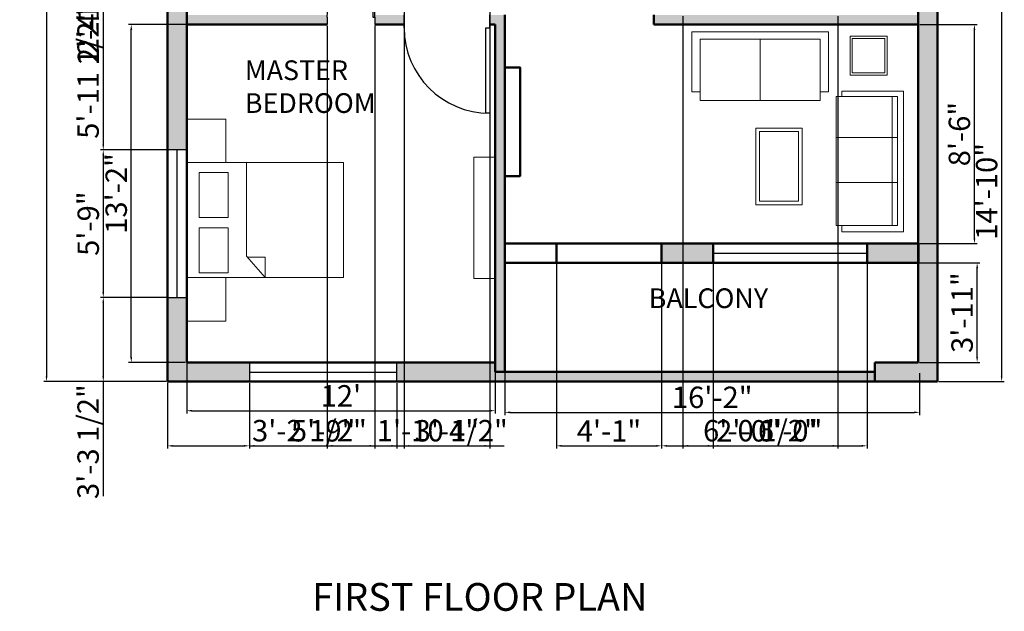
# Model space of a CAD drawing. Units: inches. Extents: x 1344 to 2521, y 3236 to 4924.
# Tile 1 of 14: x 1344 to 1805, y 3240 to 3517. Entities that reach past the tile are written whole.
import ezdxf

# ---------------------------------------------------------------- set-up
doc = ezdxf.new("R2010")
doc.units = ezdxf.units.IN
for name, color, linetype, lineweight in [('A-ANNO-DIMS', 2, 'Continuous', 18), ('A-ANNO-TEXT', 7, 'Continuous', 25), ('A-AREA-IDEN', 3, 'Continuous', 18), ('A-DOOR', 50, 'Continuous', 25), ('A-FURN', 130, 'Continuous', 18), ('A-GLAZ', 150, 'Continuous', 25), ('A-WALL', 31, 'Continuous', 50), ('A-WALL-PATT', 8, 'Continuous', 13)]:
    doc.layers.add(name, color=color, linetype=linetype, lineweight=lineweight)
doc.styles.get("Standard").update_dxf_attribs({"font": 'arial.ttf'})
doc.dimstyles.new('ISO-25', dxfattribs={"dimtxt": 10, "dimasz": 2.5, "dimexe": 1.25, "dimexo": 0.625, "dimtad": 1, "dimdec": 0, "dimlunit": 4, "dimtxsty": 'Standard', "dimcen": 2.5, "dimadec": 0, "dimazin": 0, "dimtfac": 1, "dimtdec": 0, "dimtmove": 0, "dimatfit": 3, "dimfxl": 1, "dimarcsym": 0})

# ---------------------------------------------------------------- blocks, each defined once
blk = doc.blocks.new('*U2')
for p, q in [((0, 0), (0, -6)), ((40, 0), (40, -6))]:
    blk.add_line(p, q)
blk.add_lwpolyline([(0, 0), (0, 40), (1.75, 40), (1.75, 0)], close=True)
blk.add_arc((0, 0), 40, 0, 90)
blk = doc.blocks.new('*D36')
at = {"layer": 'A-ANNO-DIMS', "color": 0, "lineweight": -2, "transparency": 16777216}
for p, q in [((1412.89, 3763.43), (1355.74, 3763.43)), ((1356.99, 3760.93), (1356.99, 3350.01)), ((1412.89, 3347.51), (1355.74, 3347.51))]:
    blk.add_line(p, q, dxfattribs=at)
at = {"layer": 'A-ANNO-DIMS', "color": 0, "lineweight": 100, "transparency": 16777216}
for points in [[(1356.58, 3760.93), (1357.41, 3760.93), (1356.99, 3763.43)], [(1356.58, 3350.01), (1357.41, 3350.01), (1356.99, 3347.51)]]:
    blk.add_solid(points, dxfattribs=at)
at = {"layer": 'Defpoints', "color": 0, "lineweight": 100, "transparency": 16777216}
for p in [(1413.52, 3763.43), (1356.99, 3347.51), (1413.52, 3347.51)]:
    blk.add_point(p, dxfattribs=at)
at = {"layer": 'A-ANNO-DIMS', "color": 0, "transparency": 16777216, "insert": (1351.26, 3555.47), "char_height": 10, "attachment_point": 5, "rotation": 90}
blk.add_mtext('34\'-8"', dxfattribs=at)
blk = doc.blocks.new('*D37')
at = {"layer": 'A-ANNO-DIMS', "color": 0, "lineweight": -2, "transparency": 16777216}
for p, q in [((1421.89, 3514.45), (1395.36, 3514.45)), ((1396.61, 3358.97), (1396.61, 3511.95)), ((1421.77, 3356.47), (1395.36, 3356.47))]:
    blk.add_line(p, q, dxfattribs=at)
at = {"layer": 'A-ANNO-DIMS', "color": 0, "lineweight": 100, "transparency": 16777216}
for points in [[(1396.19, 3511.95), (1397.03, 3511.95), (1396.61, 3514.45)], [(1396.19, 3358.97), (1397.03, 3358.97), (1396.61, 3356.47)]]:
    blk.add_solid(points, dxfattribs=at)
at = {"layer": 'Defpoints', "color": 0, "lineweight": 100, "transparency": 16777216}
for p in [(1396.61, 3514.45), (1422.52, 3514.45), (1422.4, 3356.47)]:
    blk.add_point(p, dxfattribs=at)
at = {"layer": 'A-ANNO-DIMS', "color": 0, "transparency": 16777216, "insert": (1390.87, 3435.46), "char_height": 10, "attachment_point": 5, "rotation": 90}
blk.add_mtext('13\'-2"', dxfattribs=at)
blk = doc.blocks.new('*D38')
at = {"layer": 'A-ANNO-DIMS', "color": 0, "lineweight": -2, "transparency": 16777216}
for p, q in [((1422.52, 3355.85), (1422.52, 3332.65)), ((1566.75, 3355.85), (1566.75, 3332.65)), ((1425.02, 3333.9), (1564.25, 3333.9))]:
    blk.add_line(p, q, dxfattribs=at)
at = {"layer": 'A-ANNO-DIMS', "color": 0, "lineweight": 100, "transparency": 16777216}
for points in [[(1425.02, 3334.32), (1425.02, 3333.48), (1422.52, 3333.9)], [(1564.25, 3334.32), (1564.25, 3333.48), (1566.75, 3333.9)]]:
    blk.add_solid(points, dxfattribs=at)
at = {"layer": 'Defpoints', "color": 0, "lineweight": 100, "transparency": 16777216}
for p in [(1422.52, 3356.47), (1566.75, 3356.47), (1566.75, 3333.9)]:
    blk.add_point(p, dxfattribs=at)
at = {"layer": 'A-ANNO-DIMS', "color": 0, "transparency": 16777216, "insert": (1494.63, 3339.55), "char_height": 10, "attachment_point": 5}
blk.add_mtext("12'", dxfattribs=at)
blk = doc.blocks.new('*D39')
at = {"layer": 'A-ANNO-DIMS', "color": 0, "lineweight": -2, "transparency": 16777216}
for p, q in [((1571.25, 3351.39), (1571.25, 3331.88)), ((1765.18, 3351.39), (1765.18, 3331.88)), ((1573.75, 3333.13), (1762.68, 3333.13))]:
    blk.add_line(p, q, dxfattribs=at)
at = {"layer": 'A-ANNO-DIMS', "color": 0, "lineweight": 100, "transparency": 16777216}
for points in [[(1573.75, 3333.55), (1573.75, 3332.72), (1571.25, 3333.13)], [(1762.68, 3333.55), (1762.68, 3332.72), (1765.18, 3333.13)]]:
    blk.add_solid(points, dxfattribs=at)
at = {"layer": 'Defpoints', "color": 0, "lineweight": 100, "transparency": 16777216}
for p in [(1571.25, 3352.01), (1765.18, 3352.01), (1765.18, 3333.13)]:
    blk.add_point(p, dxfattribs=at)
at = {"layer": 'A-ANNO-DIMS', "color": 0, "transparency": 16777216, "insert": (1668.22, 3338.86), "char_height": 10, "attachment_point": 5}
blk.add_mtext('16\'-2"', dxfattribs=at)
blk = doc.blocks.new('*D40')
at = {"layer": 'A-ANNO-DIMS', "color": 0, "lineweight": -2, "transparency": 16777216}
for p, q in [((1765.14, 3403.01), (1793.31, 3403.01)), ((1792.06, 3359.01), (1792.06, 3400.51)), ((1765.14, 3356.51), (1793.31, 3356.51))]:
    blk.add_line(p, q, dxfattribs=at)
at = {"layer": 'A-ANNO-DIMS', "color": 0, "lineweight": 100, "transparency": 16777216}
for points in [[(1791.64, 3400.51), (1792.48, 3400.51), (1792.06, 3403.01)], [(1791.64, 3359.01), (1792.48, 3359.01), (1792.06, 3356.51)]]:
    blk.add_solid(points, dxfattribs=at)
at = {"layer": 'Defpoints', "color": 0, "lineweight": 100, "transparency": 16777216}
for p in [(1764.52, 3403.01), (1792.06, 3403.01), (1764.52, 3356.51)]:
    blk.add_point(p, dxfattribs=at)
at = {"layer": 'A-ANNO-DIMS', "color": 0, "transparency": 16777216, "insert": (1786.33, 3379.76), "char_height": 10, "attachment_point": 5, "rotation": 90}
blk.add_mtext('3\'-11"', dxfattribs=at)
blk = doc.blocks.new('*D41')
at = {"layer": 'A-ANNO-DIMS', "color": 0, "lineweight": -2, "transparency": 16777216}
for p, q in [((1765.35, 3514.45), (1792.05, 3514.45)), ((1790.8, 3414.51), (1790.8, 3511.95)), ((1765.35, 3412.01), (1792.05, 3412.01))]:
    blk.add_line(p, q, dxfattribs=at)
at = {"layer": 'A-ANNO-DIMS', "color": 0, "lineweight": 100, "transparency": 16777216}
for points in [[(1790.38, 3511.95), (1791.22, 3511.95), (1790.8, 3514.45)], [(1790.38, 3414.51), (1791.22, 3414.51), (1790.8, 3412.01)]]:
    blk.add_solid(points, dxfattribs=at)
at = {"layer": 'Defpoints', "color": 0, "lineweight": 100, "transparency": 16777216}
for p in [(1764.72, 3514.45), (1790.8, 3514.45), (1764.72, 3412.01)]:
    blk.add_point(p, dxfattribs=at)
at = {"layer": 'A-ANNO-DIMS', "color": 0, "transparency": 16777216, "insert": (1785.07, 3463.23), "char_height": 10, "attachment_point": 5, "rotation": 90}
blk.add_mtext('8\'-6"', dxfattribs=at)
blk = doc.blocks.new('BED-DOUBLE')
for p, q in [((27.95, 53.78), (27.95, 9.98)), ((27.95, 9.98), (36.68, 0)), ((36.68, 9.56), (28.32, 9.56)), ((36.68, 0), (36.68, 9.56))]:
    blk.add_line(p, q)
for points in [[(0, 0), (73.35, 0), (73.35, 53.78), (0, 53.78)], [(5.91, 28.08), (19.39, 28.08), (19.39, 49.13), (5.91, 49.13)], [(5.91, 2.27), (19.39, 2.27), (19.39, 23.31), (5.91, 23.31)]]:
    blk.add_lwpolyline(points, close=True)
blk = doc.blocks.new('*D164')
at = {"layer": 'A-ANNO-DIMS', "color": 0, "lineweight": -2, "transparency": 16777216}
for p, q in [((1412.89, 3580.89), (1382.27, 3580.89)), ((1383.52, 3578.39), (1383.52, 3557.95)), ((1412.89, 3555.45), (1382.27, 3555.45)), ((1383.52, 3555.45), (1383.52, 3501.65))]:
    blk.add_line(p, q, dxfattribs=at)
at = {"layer": 'A-ANNO-DIMS', "color": 0, "lineweight": 100, "transparency": 16777216}
for points in [[(1383.1, 3578.39), (1383.93, 3578.39), (1383.52, 3580.89)], [(1383.1, 3557.95), (1383.93, 3557.95), (1383.52, 3555.45)]]:
    blk.add_solid(points, dxfattribs=at)
at = {"layer": 'Defpoints', "color": 0, "lineweight": 100, "transparency": 16777216}
for p in [(1413.52, 3580.89), (1383.52, 3555.45), (1413.52, 3555.45)]:
    blk.add_point(p, dxfattribs=at)
at = {"layer": 'A-ANNO-DIMS', "color": 0, "transparency": 16777216, "insert": (1377.72, 3527.3), "char_height": 10, "attachment_point": 5, "rotation": 90}
blk.add_mtext('2\'-1 1/2"', dxfattribs=at)
blk = doc.blocks.new('*D165')
at = {"layer": 'A-ANNO-DIMS', "color": 0, "lineweight": -2, "transparency": 16777216}
for p, q in [((1412.89, 3555.45), (1382.27, 3555.45)), ((1383.52, 3552.95), (1383.52, 3529.97)), ((1412.89, 3527.47), (1382.27, 3527.47)), ((1383.52, 3527.47), (1383.52, 3496.97))]:
    blk.add_line(p, q, dxfattribs=at)
at = {"layer": 'A-ANNO-DIMS', "color": 0, "lineweight": 100, "transparency": 16777216}
for points in [[(1383.1, 3552.95), (1383.93, 3552.95), (1383.52, 3555.45)], [(1383.1, 3529.97), (1383.93, 3529.97), (1383.52, 3527.47)]]:
    blk.add_solid(points, dxfattribs=at)
at = {"layer": 'Defpoints', "color": 0, "lineweight": 100, "transparency": 16777216}
for p in [(1413.52, 3555.45), (1383.52, 3527.47), (1413.52, 3527.47)]:
    blk.add_point(p, dxfattribs=at)
at = {"layer": 'A-ANNO-DIMS', "color": 0, "transparency": 16777216, "insert": (1377.87, 3510.97), "char_height": 10, "attachment_point": 5, "rotation": 90}
blk.add_mtext('2\'-4"', dxfattribs=at)
blk = doc.blocks.new('*D166')
at = {"layer": 'A-ANNO-DIMS', "color": 0, "lineweight": -2, "transparency": 16777216}
for p, q in [((1412.89, 3527.47), (1382.27, 3527.47)), ((1383.52, 3524.97), (1383.52, 3458.32)), ((1412.89, 3455.82), (1382.27, 3455.82))]:
    blk.add_line(p, q, dxfattribs=at)
at = {"layer": 'A-ANNO-DIMS', "color": 0, "lineweight": 100, "transparency": 16777216}
for points in [[(1383.1, 3524.97), (1383.93, 3524.97), (1383.52, 3527.47)], [(1383.1, 3458.32), (1383.93, 3458.32), (1383.52, 3455.82)]]:
    blk.add_solid(points, dxfattribs=at)
at = {"layer": 'Defpoints', "color": 0, "lineweight": 100, "transparency": 16777216}
for p in [(1413.52, 3527.47), (1383.52, 3455.82), (1413.52, 3455.82)]:
    blk.add_point(p, dxfattribs=at)
at = {"layer": 'A-ANNO-DIMS', "color": 0, "transparency": 16777216, "insert": (1377.72, 3491.65), "char_height": 10, "attachment_point": 5, "rotation": 90}
blk.add_mtext('5\'-11 1/2"', dxfattribs=at)
blk = doc.blocks.new('*D167')
at = {"layer": 'A-ANNO-DIMS', "color": 0, "lineweight": -2, "transparency": 16777216}
for p, q in [((1412.89, 3455.82), (1382.27, 3455.82)), ((1383.52, 3453.32), (1383.52, 3389.4)), ((1412.89, 3386.9), (1382.27, 3386.9))]:
    blk.add_line(p, q, dxfattribs=at)
at = {"layer": 'A-ANNO-DIMS', "color": 0, "lineweight": 100, "transparency": 16777216}
for points in [[(1383.1, 3453.32), (1383.93, 3453.32), (1383.52, 3455.82)], [(1383.1, 3389.4), (1383.93, 3389.4), (1383.52, 3386.9)]]:
    blk.add_solid(points, dxfattribs=at)
at = {"layer": 'Defpoints', "color": 0, "lineweight": 100, "transparency": 16777216}
for p in [(1413.52, 3455.82), (1383.52, 3386.9), (1413.52, 3386.9)]:
    blk.add_point(p, dxfattribs=at)
at = {"layer": 'A-ANNO-DIMS', "color": 0, "transparency": 16777216, "insert": (1377.79, 3421.36), "char_height": 10, "attachment_point": 5, "rotation": 90}
blk.add_mtext('5\'-9"', dxfattribs=at)
blk = doc.blocks.new('*D168')
at = {"layer": 'A-ANNO-DIMS', "color": 0, "lineweight": -2, "transparency": 16777216}
for p, q in [((1412.89, 3386.9), (1382.27, 3386.9)), ((1383.52, 3384.4), (1383.52, 3350.01)), ((1412.89, 3347.51), (1382.27, 3347.51)), ((1383.52, 3347.51), (1383.52, 3293.88))]:
    blk.add_line(p, q, dxfattribs=at)
at = {"layer": 'A-ANNO-DIMS', "color": 0, "lineweight": 100, "transparency": 16777216}
for points in [[(1383.1, 3384.4), (1383.93, 3384.4), (1383.52, 3386.9)], [(1383.1, 3350.01), (1383.93, 3350.01), (1383.52, 3347.51)]]:
    blk.add_solid(points, dxfattribs=at)
at = {"layer": 'Defpoints', "color": 0, "lineweight": 100, "transparency": 16777216}
for p in [(1413.52, 3386.9), (1383.52, 3347.51), (1413.52, 3347.51)]:
    blk.add_point(p, dxfattribs=at)
at = {"layer": 'A-ANNO-DIMS', "color": 0, "transparency": 16777216, "insert": (1377.72, 3319.45), "char_height": 10, "attachment_point": 5, "rotation": 90}
blk.add_mtext('3\'-3 1/2"', dxfattribs=at)
blk = doc.blocks.new('*D171')
at = {"layer": 'A-ANNO-DIMS', "color": 0, "lineweight": -2, "transparency": 16777216}
for p, q in [((1774.14, 3525.36), (1804.77, 3525.36)), ((1803.52, 3522.86), (1803.52, 3350.01)), ((1774.14, 3347.51), (1804.77, 3347.51))]:
    blk.add_line(p, q, dxfattribs=at)
at = {"layer": 'A-ANNO-DIMS', "color": 0, "lineweight": 100, "transparency": 16777216}
for points in [[(1803.1, 3522.86), (1803.93, 3522.86), (1803.52, 3525.36)], [(1803.1, 3350.01), (1803.93, 3350.01), (1803.52, 3347.51)]]:
    blk.add_solid(points, dxfattribs=at)
at = {"layer": 'Defpoints', "color": 0, "lineweight": 100, "transparency": 16777216}
for p in [(1773.52, 3525.36), (1773.52, 3347.51), (1803.52, 3347.51)]:
    blk.add_point(p, dxfattribs=at)
at = {"layer": 'A-ANNO-DIMS', "color": 0, "transparency": 16777216, "insert": (1797.79, 3436.44), "char_height": 10, "attachment_point": 5, "rotation": 90}
blk.add_mtext('14\'-10"', dxfattribs=at)
blk = doc.blocks.new('*D172')
at = {"layer": 'A-ANNO-DIMS', "color": 0, "lineweight": -2, "transparency": 16777216}
for p, q in [((1413.52, 3346.89), (1413.52, 3316.22)), ((1451.85, 3346.85), (1451.85, 3316.22)), ((1416.02, 3317.47), (1449.35, 3317.47)), ((1451.85, 3317.47), (1505.48, 3317.47))]:
    blk.add_line(p, q, dxfattribs=at)
at = {"layer": 'A-ANNO-DIMS', "color": 0, "lineweight": 100, "transparency": 16777216}
for points in [[(1416.02, 3317.89), (1416.02, 3317.06), (1413.52, 3317.47)], [(1449.35, 3317.89), (1449.35, 3317.06), (1451.85, 3317.47)]]:
    blk.add_solid(points, dxfattribs=at)
at = {"layer": 'Defpoints', "color": 0, "lineweight": 100, "transparency": 16777216}
for p in [(1413.52, 3347.51), (1451.85, 3347.47), (1451.85, 3317.47)]:
    blk.add_point(p, dxfattribs=at)
at = {"layer": 'A-ANNO-DIMS', "color": 0, "transparency": 16777216, "insert": (1479.91, 3323.27), "char_height": 10, "attachment_point": 5}
blk.add_mtext('3\'-2 1/2"', dxfattribs=at)
blk = doc.blocks.new('*D173')
at = {"layer": 'A-ANNO-DIMS', "color": 0, "lineweight": -2, "transparency": 16777216}
for p, q in [((1451.85, 3346.85), (1451.85, 3316.22)), ((1520.77, 3346.85), (1520.77, 3316.22)), ((1454.35, 3317.47), (1518.27, 3317.47))]:
    blk.add_line(p, q, dxfattribs=at)
at = {"layer": 'A-ANNO-DIMS', "color": 0, "lineweight": 100, "transparency": 16777216}
for points in [[(1454.35, 3317.89), (1454.35, 3317.06), (1451.85, 3317.47)], [(1518.27, 3317.89), (1518.27, 3317.06), (1520.77, 3317.47)]]:
    blk.add_solid(points, dxfattribs=at)
at = {"layer": 'Defpoints', "color": 0, "lineweight": 100, "transparency": 16777216}
for p in [(1451.85, 3347.47), (1520.77, 3347.47), (1520.77, 3317.47)]:
    blk.add_point(p, dxfattribs=at)
at = {"layer": 'A-ANNO-DIMS', "color": 0, "transparency": 16777216, "insert": (1486.31, 3323.2), "char_height": 10, "attachment_point": 5}
blk.add_mtext('5\'-9"', dxfattribs=at)
blk = doc.blocks.new('*D175')
at = {"layer": 'A-ANNO-DIMS', "color": 0, "lineweight": -2, "transparency": 16777216}
for p, q in [((1524.17, 3619.06), (1524.17, 3316.22)), ((1564.17, 3619.06), (1564.17, 3316.22)), ((1526.67, 3317.47), (1561.67, 3317.47))]:
    blk.add_line(p, q, dxfattribs=at)
at = {"layer": 'A-ANNO-DIMS', "color": 0, "lineweight": 100, "transparency": 16777216}
for points in [[(1526.67, 3317.89), (1526.67, 3317.06), (1524.17, 3317.47)], [(1561.67, 3317.89), (1561.67, 3317.06), (1564.17, 3317.47)]]:
    blk.add_solid(points, dxfattribs=at)
at = {"layer": 'Defpoints', "color": 0, "lineweight": 100, "transparency": 16777216}
for p in [(1524.17, 3619.69), (1564.17, 3619.69), (1564.17, 3317.47)]:
    blk.add_point(p, dxfattribs=at)
at = {"layer": 'A-ANNO-DIMS', "color": 0, "transparency": 16777216, "insert": (1544.17, 3323.21), "char_height": 10, "attachment_point": 5}
blk.add_mtext('3\'-4"', dxfattribs=at)
blk = doc.blocks.new('*D176')
at = {"layer": 'A-ANNO-DIMS', "color": 0, "lineweight": -2, "transparency": 16777216}
for p, q in [((1488.21, 3513.82), (1488.21, 3316.22)), ((1510.55, 3513.82), (1510.55, 3316.22)), ((1490.71, 3317.47), (1508.05, 3317.47)), ((1510.55, 3317.47), (1571.01, 3317.47))]:
    blk.add_line(p, q, dxfattribs=at)
at = {"layer": 'A-ANNO-DIMS', "color": 0, "lineweight": 100, "transparency": 16777216}
for points in [[(1490.71, 3317.89), (1490.71, 3317.06), (1488.21, 3317.47)], [(1508.05, 3317.89), (1508.05, 3317.06), (1510.55, 3317.47)]]:
    blk.add_solid(points, dxfattribs=at)
at = {"layer": 'Defpoints', "color": 0, "lineweight": 100, "transparency": 16777216}
for p in [(1488.21, 3514.45), (1510.55, 3514.45), (1510.55, 3317.47)]:
    blk.add_point(p, dxfattribs=at)
at = {"layer": 'A-ANNO-DIMS', "color": 0, "transparency": 16777216, "insert": (1542.03, 3323.27), "char_height": 10, "attachment_point": 5}
blk.add_mtext('1\'-10 1/2"', dxfattribs=at)
blk = doc.blocks.new('*D181')
at = {"layer": 'A-ANNO-DIMS', "color": 0, "lineweight": -2, "transparency": 16777216}
for p, q in [((1595.35, 3411.39), (1595.35, 3316.22)), ((1644.53, 3411.39), (1644.53, 3316.22)), ((1597.85, 3317.47), (1642.03, 3317.47))]:
    blk.add_line(p, q, dxfattribs=at)
at = {"layer": 'A-ANNO-DIMS', "color": 0, "lineweight": 100, "transparency": 16777216}
for points in [[(1597.85, 3317.89), (1597.85, 3317.06), (1595.35, 3317.47)], [(1642.03, 3317.89), (1642.03, 3317.06), (1644.53, 3317.47)]]:
    blk.add_solid(points, dxfattribs=at)
at = {"layer": 'Defpoints', "color": 0, "lineweight": 100, "transparency": 16777216}
for p in [(1595.35, 3412.01), (1644.53, 3412.01), (1644.53, 3317.47)]:
    blk.add_point(p, dxfattribs=at)
at = {"layer": 'A-ANNO-DIMS', "color": 0, "transparency": 16777216, "insert": (1619.94, 3323.12), "char_height": 10, "attachment_point": 5}
blk.add_mtext('4\'-1"', dxfattribs=at)
blk = doc.blocks.new('*D182')
at = {"layer": 'A-ANNO-DIMS', "color": 0, "lineweight": -2, "transparency": 16777216}
for p, q in [((1644.53, 3411.39), (1644.53, 3316.22)), ((1668.63, 3411.39), (1668.63, 3316.22)), ((1647.03, 3317.47), (1666.13, 3317.47)), ((1668.63, 3317.47), (1699.13, 3317.47))]:
    blk.add_line(p, q, dxfattribs=at)
at = {"layer": 'A-ANNO-DIMS', "color": 0, "lineweight": 100, "transparency": 16777216}
for points in [[(1647.03, 3317.89), (1647.03, 3317.06), (1644.53, 3317.47)], [(1666.13, 3317.89), (1666.13, 3317.06), (1668.63, 3317.47)]]:
    blk.add_solid(points, dxfattribs=at)
at = {"layer": 'Defpoints', "color": 0, "lineweight": 100, "transparency": 16777216}
for p in [(1644.53, 3412.01), (1668.63, 3412.01), (1668.63, 3317.47)]:
    blk.add_point(p, dxfattribs=at)
at = {"layer": 'A-ANNO-DIMS', "color": 0, "transparency": 16777216, "insert": (1685.13, 3323.2), "char_height": 10, "attachment_point": 5}
blk.add_mtext('2\'-0"', dxfattribs=at)
blk = doc.blocks.new('*D183')
at = {"layer": 'A-ANNO-DIMS', "color": 0, "lineweight": -2, "transparency": 16777216}
for p, q in [((1668.63, 3411.39), (1668.63, 3316.22)), ((1740.62, 3411.39), (1740.62, 3316.22)), ((1671.13, 3317.47), (1738.12, 3317.47))]:
    blk.add_line(p, q, dxfattribs=at)
at = {"layer": 'A-ANNO-DIMS', "color": 0, "lineweight": 100, "transparency": 16777216}
for points in [[(1671.13, 3317.89), (1671.13, 3317.06), (1668.63, 3317.47)], [(1738.12, 3317.89), (1738.12, 3317.06), (1740.62, 3317.47)]]:
    blk.add_solid(points, dxfattribs=at)
at = {"layer": 'Defpoints', "color": 0, "lineweight": 100, "transparency": 16777216}
for p in [(1668.63, 3412.01), (1740.62, 3412.01), (1740.62, 3317.47)]:
    blk.add_point(p, dxfattribs=at)
at = {"layer": 'A-ANNO-DIMS', "color": 0, "transparency": 16777216, "insert": (1704.62, 3323.2), "char_height": 10, "attachment_point": 5}
blk.add_mtext('6\'-0"', dxfattribs=at)
blk = doc.blocks.new('*D184')
at = {"layer": 'A-ANNO-DIMS', "color": 0, "lineweight": -2, "transparency": 16777216}
for p, q in [((1654.54, 3518.32), (1654.54, 3316.22)), ((1727.01, 3518.32), (1727.01, 3316.22)), ((1657.04, 3317.47), (1724.51, 3317.47))]:
    blk.add_line(p, q, dxfattribs=at)
at = {"layer": 'A-ANNO-DIMS', "color": 0, "lineweight": 100, "transparency": 16777216}
for points in [[(1657.04, 3317.89), (1657.04, 3317.06), (1654.54, 3317.47)], [(1724.51, 3317.89), (1724.51, 3317.06), (1727.01, 3317.47)]]:
    blk.add_solid(points, dxfattribs=at)
at = {"layer": 'Defpoints', "color": 0, "lineweight": 100, "transparency": 16777216}
for p in [(1654.54, 3518.95), (1727.01, 3518.95), (1727.01, 3317.47)]:
    blk.add_point(p, dxfattribs=at)
at = {"layer": 'A-ANNO-DIMS', "color": 0, "transparency": 16777216, "insert": (1690.78, 3323.27), "char_height": 10, "attachment_point": 5}
blk.add_mtext('6\'-0 1/2"', dxfattribs=at)

msp = doc.modelspace()

# ---------------------------------------------------------------- hatches: boundary and pattern name
at = {"layer": 'A-WALL-PATT'}
h = msp.add_hatch(color=256, dxfattribs=at)
h.dxf.hatch_style = 1
h.paths.add_polyline_path([(1451.85, 3356.47), (1422.52, 3356.47), (1422.52, 3386.9), (1413.52, 3386.9), (1413.52, 3347.51), (1451.85, 3347.51)])
h.paths.add_polyline_path([(1744.16, 3352.01), (1566.75, 3352.01), (1566.75, 3356.47), (1544.82, 3356.47), (1520.77, 3356.47), (1520.77, 3347.51), (1744.16, 3347.51)])
h.paths.add_polyline_path([(1773.52, 3525.36), (1764.52, 3525.36), (1764.52, 3497.27), (1764.52, 3412.01), (1764.72, 3412.01), (1764.72, 3403.01), (1764.52, 3403.01), (1764.52, 3356.51), (1744.16, 3356.51), (1744.16, 3347.51), (1773.52, 3347.51)])
h.paths.add_polyline_path([(1764.52, 3412.01), (1740.62, 3412.01), (1740.62, 3403.01), (1764.52, 3403.01)])
h.paths.add_polyline_path([(1668.63, 3412.01), (1644.53, 3412.01), (1644.53, 3403.01), (1668.63, 3403.01)])
h.paths.add_polyline_path([(1571.25, 3514.45), (1571.25, 3518.95), (1564.17, 3518.95), (1564.17, 3514.45), (1566.75, 3514.45), (1566.75, 3352.01), (1571.25, 3352.01)])
h.paths.add_polyline_path([(1422.52, 3527.47), (1413.52, 3527.47), (1413.52, 3455.82), (1422.52, 3455.82), (1422.52, 3470.24)])
h.paths.add_polyline_path([(1488.21, 3517.8, -0.012876), (1488.24, 3518.95), (1422.52, 3518.95), (1422.52, 3514.45), (1488.21, 3514.45)])
h.paths.add_polyline_path([(1524.17, 3518.95), (1510.55, 3518.95), (1510.55, 3517.8), (1510.55, 3514.45), (1524.17, 3514.45)])
h.paths.add_polyline_path([(1764.52, 3518.95), (1640.94, 3518.95), (1640.94, 3514.45), (1764.52, 3514.45)])
h.paths.add_polyline_path([(1764.52, 3610.02), (1645.44, 3610.02), (1645.44, 3605.52), (1764.52, 3605.52)])
h.paths.add_polyline_path([(1645.44, 3610.02), (1640.94, 3610.02), (1640.94, 3605.52), (1645.44, 3605.52)])
h.paths.add_polyline_path([(1422.52, 3580.89), (1413.52, 3580.89), (1413.52, 3555.45), (1422.52, 3555.45)])
h.paths.add_polyline_path([(1513.17, 3573.32), (1505.17, 3573.32), (1505.17, 3573.28), (1475.67, 3573.28), (1422.52, 3573.32), (1422.52, 3568.82), (1513.17, 3568.82)])
h.paths.add_polyline_path([(1635.28, 3376.69), (1701.38, 3376.69), (1701.38, 3395.67), (1635.28, 3395.67)], flags=9)
h.paths.add_polyline_path([(1526.07, 3560.64), (1635.07, 3560.64), (1635.07, 3579.62), (1526.07, 3579.62)], flags=9)
h.paths.add_polyline_path([(1666.39, 3730.09), (1741.06, 3730.09), (1741.06, 3749.07), (1666.39, 3749.07)], flags=9)
h.paths.add_polyline_path([(1446.44, 3467.76), (1517.54, 3467.76), (1517.54, 3502.26), (1446.44, 3502.26)], flags=9)
h.paths.add_polyline_path([(1429.07, 3520.24), (1478.72, 3520.24), (1478.72, 3539.22), (1429.07, 3539.22)], flags=9)
h.paths.add_polyline_path([(1425.85, 3603.57), (1475.5, 3603.57), (1475.5, 3622.55), (1425.85, 3622.55)], flags=9)
h.paths.add_polyline_path([(1570.93, 3699.42), (1620.58, 3699.42), (1620.58, 3718.41), (1570.93, 3718.41)], flags=9)
h.paths.add_polyline_path([(1447.04, 3718.72), (1518.14, 3718.72), (1518.14, 3753.22), (1447.04, 3753.22)], flags=9)

# ---------------------------------------------------------------- linework, layer by layer
at = {"layer": 'A-FURN'}
for p, q in [((1658.71, 3482.9), (1658.71, 3511.03)), ((1658.71, 3511.03), (1722.65, 3511.03)), ((1722.65, 3511.03), (1722.65, 3482.9)), ((1690.66, 3478.9), (1690.66, 3507.57)), ((1662.65, 3482.9), (1658.71, 3482.9)), ((1722.65, 3482.9), (1718.66, 3482.9)), ((1728.86, 3480.84), (1728.86, 3483.3)), ((1728.86, 3483.3), (1757.6, 3483.3)), ((1752.39, 3420.48), (1752.39, 3480.84)), ((1757.6, 3417.54), (1757.6, 3483.3)), ((1754.8, 3461.66), (1726.18, 3461.66)), ((1754.8, 3440.51), (1726.18, 3440.51)), ((1728.86, 3417.54), (1728.86, 3420.48)), ((1757.6, 3417.54), (1728.86, 3417.54))]:
    msp.add_line(p, q, dxfattribs=at)
for points in [[(1732.64, 3490.77), (1749.93, 3490.77), (1749.93, 3508.95), (1732.64, 3508.95)], [(1733.67, 3491.79), (1748.91, 3491.79), (1748.91, 3507.93), (1733.67, 3507.93)], [(1718.66, 3478.9), (1662.65, 3478.9), (1662.65, 3507.57), (1718.66, 3507.57)], [(1754.8, 3480.84), (1726.18, 3480.84), (1726.18, 3420.48), (1754.8, 3420.48)], [(1422.52, 3449.9), (1440.75, 3449.9), (1440.75, 3470.24), (1422.52, 3470.24)], [(1710.24, 3465.98), (1688.62, 3465.98), (1688.62, 3430.18), (1710.24, 3430.18)], [(1708.61, 3464.35), (1690.25, 3464.35), (1690.25, 3431.8), (1708.61, 3431.8)], [(1566.75, 3452.39), (1556.79, 3452.39), (1556.79, 3395.65), (1566.75, 3395.65)], [(1422.52, 3375.77), (1440.75, 3375.77), (1440.75, 3396.12), (1422.52, 3396.12)]]:
    msp.add_lwpolyline(points, close=True, dxfattribs=at)
at = {"layer": 'A-GLAZ'}
for p, q in [((1418.02, 3386.9), (1418.02, 3455.82)), ((1668.63, 3407.51), (1740.62, 3407.51)), ((1451.85, 3351.97), (1520.77, 3351.97))]:
    msp.add_line(p, q, dxfattribs=at)
for points in [[(1413.52, 3386.9), (1422.52, 3386.9), (1422.52, 3455.82), (1413.52, 3455.82)], [(1451.85, 3356.47), (1451.85, 3347.47), (1520.77, 3347.47), (1520.77, 3356.47)]]:
    msp.add_lwpolyline(points, close=True, dxfattribs=at)
at = {"layer": 'A-WALL'}
for p, q in [((1764.52, 3533.27), (1764.52, 3497.27)), ((1571.25, 3514.45), (1571.25, 3518.95)), ((1640.94, 3518.95), (1640.94, 3514.45)), ((1422.52, 3514.45), (1488.21, 3514.45)), ((1510.55, 3514.45), (1524.17, 3514.45)), ((1564.17, 3514.45), (1566.75, 3514.45)), ((1566.75, 3514.45), (1566.75, 3352.01)), ((1571.25, 3514.45), (1571.25, 3352.01)), ((1640.94, 3514.45), (1764.52, 3514.45)), ((1764.52, 3397.36), (1764.52, 3433.36)), ((1764.52, 3412.01), (1571.25, 3412.01)), ((1764.52, 3403.01), (1571.25, 3403.01)), ((1422.4, 3356.47), (1544.82, 3356.47)), ((1544.82, 3356.47), (1566.75, 3356.47)), ((1744.16, 3347.51), (1744.16, 3356.51)), ((1744.16, 3356.51), (1764.52, 3356.51)), ((1566.75, 3352.01), (1744.16, 3352.01)), ((1579.5, 3352.01), (1589.02, 3352.01)), ((1726.01, 3352.01), (1726.01, 3352.11)), ((1422.52, 3347.51), (1413.52, 3347.51)), ((1413.52, 3347.51), (1773.52, 3347.51)), ((1422.52, 3347.51), (1544.94, 3347.51)), ((1579.5, 3347.51), (1589.02, 3347.51)), ((1773.52, 3347.51), (1744.16, 3347.51))]:
    msp.add_line(p, q, dxfattribs=at)
for points in [[(1773.52, 3347.51), (1773.52, 3763.43), (1413.52, 3763.43), (1413.52, 3347.51)], [(1764.52, 3356.51), (1764.52, 3754.43), (1422.52, 3754.43), (1422.52, 3356.47)]]:
    msp.add_lwpolyline(points, dxfattribs=at)
for points in [[(1571.25, 3443.57), (1578.4, 3443.57), (1578.4, 3494.41), (1571.25, 3494.41)], [(1571.25, 3412.01), (1595.35, 3412.01), (1595.35, 3403.01), (1571.25, 3403.01)], [(1644.53, 3412.01), (1668.63, 3412.01), (1668.63, 3403.01), (1644.53, 3403.01)], [(1740.62, 3412.01), (1764.72, 3412.01), (1764.72, 3403.01), (1740.62, 3403.01)]]:
    msp.add_lwpolyline(points, close=True, dxfattribs=at)

# ---------------------------------------------------------------- block references
at = {"layer": 'A-DOOR', "xscale": -0.5583757449765673, "yscale": 0.5583757449765673, "zscale": 0.5583757449765673}
msp.add_blockref('*U2', (1510.55, 3517.8), dxfattribs=at)
at = {"layer": 'A-DOOR', "rotation": 180}
msp.add_blockref('*U2', (1564.17, 3512.95), dxfattribs=at)
at = {"layer": 'A-FURN'}
msp.add_blockref('BED-DOUBLE', (1422.52, 3396.12), dxfattribs=at)

# ---------------------------------------------------------------- texts
at = {"layer": 'A-ANNO-TEXT', "insert": (1481.16, 3253.34), "char_height": 12.9935, "attachment_point": 1}
msp.add_mtext_dynamic_manual_height_columns('FIRST FLOOR PLAN', width=2122.9296, gutter_width=64.97, heights=[0], dxfattribs=at)
at = {"layer": 'A-AREA-IDEN', "char_height": 9.211, "attachment_point": 1}
for s, insert in [('MASTER BEDROOM', (1449.7, 3497.67)), ('BALCONY', (1638.53, 3391.09))]:
    msp.add_mtext_dynamic_manual_height_columns(s, width=108.7809, gutter_width=46.06, heights=[0], dxfattribs=dict(at, insert=insert))

# ---------------------------------------------------------------- dimensions: what is measured, and where the dimension line sits
at = {"layer": 'A-ANNO-DIMS'}
dim = msp.add_linear_dim(base=(1356.99, 3347.51), p1=(1413.52, 3763.43), p2=(1413.52, 3347.51), angle=90, dimstyle='ISO-25', override={"dimclrd": 0, "dimclre": 0, "dimclrt": 0}, dxfattribs=at)
dim.commit()
dim.dimension.update_dxf_attribs({"geometry": '*D36', "text_midpoint": (1356.99, 3555.47), "dimtype": 160})
for base, p1, p2, override, picture, middle in [((1564.17, 3317.47), (1524.17, 3619.69), (1564.17, 3619.69), {"dimdec": 1, "dimlfac": 1, "dimrnd": 0, "dimzin": 1, "dimdsep": 46, "dimlunit": 4, "dimfrac": 2}, '*D175', (1544.17, 3323.21)), ((1727.01, 3317.47), (1654.54, 3518.95), (1727.01, 3518.95), {"dimdec": 1, "dimlfac": 1, "dimrnd": 0, "dimzin": 1, "dimdsep": 46, "dimlunit": 4, "dimfrac": 2}, '*D184', (1690.78, 3323.27)), ((1510.55, 3317.47), (1488.21, 3514.45), (1510.55, 3514.45), {"dimdec": 1, "dimlfac": 1, "dimrnd": 0, "dimzin": 1, "dimdsep": 46, "dimlunit": 4, "dimfrac": 2}, '*D176', (1542.03, 3323.27)), ((1644.53, 3317.47), (1595.35, 3412.01), (1644.53, 3412.01), {"dimdec": 1, "dimlfac": 1, "dimrnd": 0, "dimzin": 1, "dimdsep": 46, "dimlunit": 4, "dimfrac": 2}, '*D181', (1619.94, 3323.12)), ((1668.63, 3317.47), (1644.53, 3412.01), (1668.63, 3412.01), {"dimdec": 1, "dimlfac": 1, "dimrnd": 0, "dimzin": 1, "dimdsep": 46, "dimlunit": 4, "dimfrac": 2}, '*D182', (1685.13, 3323.2)), ((1740.62, 3317.47), (1668.63, 3412.01), (1740.62, 3412.01), {"dimdec": 1, "dimlfac": 1, "dimrnd": 0, "dimzin": 1, "dimdsep": 46, "dimlunit": 4, "dimfrac": 2}, '*D183', (1704.62, 3323.2)), ((1566.75, 3333.9), (1422.52, 3356.47), (1566.75, 3356.47), {"dimclrd": 0, "dimclre": 0, "dimclrt": 0}, '*D38', (1494.63, 3339.55)), ((1765.18, 3333.13), (1571.25, 3352.01), (1765.18, 3352.01), {"dimclrd": 0, "dimclre": 0, "dimclrt": 0}, '*D39', (1668.22, 3338.86)), ((1451.85, 3317.47), (1413.52, 3347.51), (1451.85, 3347.47), {"dimdec": 1, "dimlfac": 1, "dimrnd": 0, "dimzin": 1, "dimdsep": 46, "dimlunit": 4, "dimfrac": 2}, '*D172', (1479.91, 3323.27)), ((1520.77, 3317.47), (1451.85, 3347.47), (1520.77, 3347.47), {"dimdec": 1, "dimlfac": 1, "dimrnd": 0, "dimzin": 1, "dimdsep": 46, "dimlunit": 4, "dimfrac": 2}, '*D173', (1486.31, 3323.2))]:
    dim = msp.add_linear_dim(base=base, p1=p1, p2=p2, dimstyle='ISO-25', override=override, dxfattribs=at)
    dim.commit()
    dim.dimension.update_dxf_attribs({"geometry": picture, "text_midpoint": middle})
for base, p1, p2, override, picture, middle in [((1383.52, 3555.45), (1413.52, 3580.89), (1413.52, 3555.45), {"dimdec": 1, "dimlfac": 1, "dimrnd": 0, "dimzin": 1, "dimdsep": 46, "dimlunit": 4, "dimfrac": 2}, '*D164', (1377.72, 3527.3)), ((1383.52, 3527.47), (1413.52, 3555.45), (1413.52, 3527.47), {"dimdec": 1, "dimlfac": 1, "dimrnd": 0, "dimzin": 1, "dimdsep": 46, "dimlunit": 4, "dimfrac": 2}, '*D165', (1377.87, 3510.97)), ((1383.5178, 3455.8226), (1413.5178, 3527.4742), (1413.5178, 3455.8226), {"dimdec": 1, "dimlfac": 1, "dimrnd": 0, "dimzin": 1, "dimdsep": 46, "dimlunit": 4, "dimfrac": 2}, '*D166', (1377.7223, 3491.6484)), ((1803.5178, 3347.5114), (1773.5178, 3525.3602), (1773.5178, 3347.5114), {"dimdec": 1, "dimlfac": 1, "dimrnd": 0, "dimzin": 1, "dimdsep": 46, "dimlunit": 4, "dimfrac": 2}, '*D171', (1797.7871, 3436.4358)), ((1396.61, 3514.45), (1422.4, 3356.47), (1422.52, 3514.45), {"dimclrd": 0, "dimclre": 0, "dimclrt": 0}, '*D37', (1390.87, 3435.46)), ((1790.8, 3514.45), (1764.72, 3412.01), (1764.72, 3514.45), {"dimclrd": 0, "dimclre": 0, "dimclrt": 0}, '*D41', (1785.07, 3463.23)), ((1383.52, 3386.9), (1413.52, 3455.82), (1413.52, 3386.9), {"dimdec": 1, "dimlfac": 1, "dimrnd": 0, "dimzin": 1, "dimdsep": 46, "dimlunit": 4, "dimfrac": 2}, '*D167', (1377.79, 3421.36)), ((1792.061, 3403.0116), (1764.5178, 3356.5114), (1764.5178, 3403.0116), {"dimclrd": 0, "dimclre": 0, "dimclrt": 0}, '*D40', (1786.3268, 3379.7615)), ((1383.52, 3347.51), (1413.52, 3386.9), (1413.52, 3347.51), {"dimdec": 1, "dimlfac": 1, "dimrnd": 0, "dimzin": 1, "dimdsep": 46, "dimlunit": 4, "dimfrac": 2}, '*D168', (1377.72, 3319.45))]:
    dim = msp.add_linear_dim(base=base, p1=p1, p2=p2, angle=90, dimstyle='ISO-25', override=override, dxfattribs=at)
    dim.commit()
    dim.dimension.update_dxf_attribs({"geometry": picture, "text_midpoint": middle})

doc.saveas('drawing.dxf')
